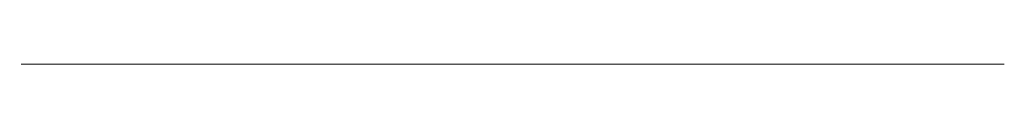
# Model space of a CAD drawing. Units: inches. Extents: x 846 to 1079, y 0 to 0.
import ezdxf

# ---------------------------------------------------------------- set-up
doc = ezdxf.new("R2010")
doc.units = ezdxf.units.IN
doc.header["$MEASUREMENT"] = 0
doc.layers.add('M-CONS', color=8, linetype='Continuous', lineweight=18)

msp = doc.modelspace()

# ---------------------------------------------------------------- linework, layer by layer
at = {"layer": 'M-CONS', "extrusion": (0, -1, 0)}
for p, q in [((977.23, 0, 538.66), (1012.52, 0, 538.66)), ((981.25, 0, 568.66), (1011.77, 0, 568.66))]:
    msp.add_line(p, q, dxfattribs=at)
for points in [[(933.75, 483.66, -0.268184), (886.07, 511.16, 1), (851.43, 491.16, 0.268121), (933.77, 443.66)], [(933.74, 483.66, -0.16796), (946.09, 479.4), (945.69, 518.86, 0.411246), (925.7, 538.66), (861.25, 538.66, -1), (861.25, 568.66, 1), (861.25, 538.66)], [(933.77, 663.66, 0.268121), (851.43, 616.16, 1), (886.07, 596.16, -0.268184), (933.75, 623.66)], [(933.75, 451.16, 1.000321), (933.75, 476.16, -0.268121), (879.58, 507.41, 1), (857.93, 494.91, 0.268121), (933.76, 451.16)], [(933.76, 656.16, 0.268121), (857.93, 612.41, 1), (879.58, 599.91, -0.268121), (933.75, 631.16, -0.000032), (933.75, 631.16)], [(933.74, 623.66, 0.16796), (946.09, 627.92), (945.69, 588.45, -0.411246), (925.7, 568.66), (861.25, 568.66)], [(933.75, 443.66, 0.417188), (953.75, 463.86), (953.2, 518.45, -0.417188), (973.2, 538.66), (981.25, 538.66)], [(981.25, 568.66), (973.2, 568.66, -0.417188), (953.2, 588.86), (953.75, 643.45, 0.417188), (933.75, 663.66)]]:
    msp.add_lwpolyline(points, format="xyb", dxfattribs=at)
for centre, radius in [((861.25, 553.66), 7.5), ((901.25, 553.66), 7.5), ((941.25, 553.66), 7.5), ((981.25, 553.66), 7.5), ((1043.75, 554.45), 35), ((1043.75, 554.45), 25)]:
    msp.add_circle(centre, radius, dxfattribs=at)
msp.add_arc((933.75, 643.66), 12.5, 269.9633, 90, dxfattribs=at)

doc.saveas('drawing.dxf')
